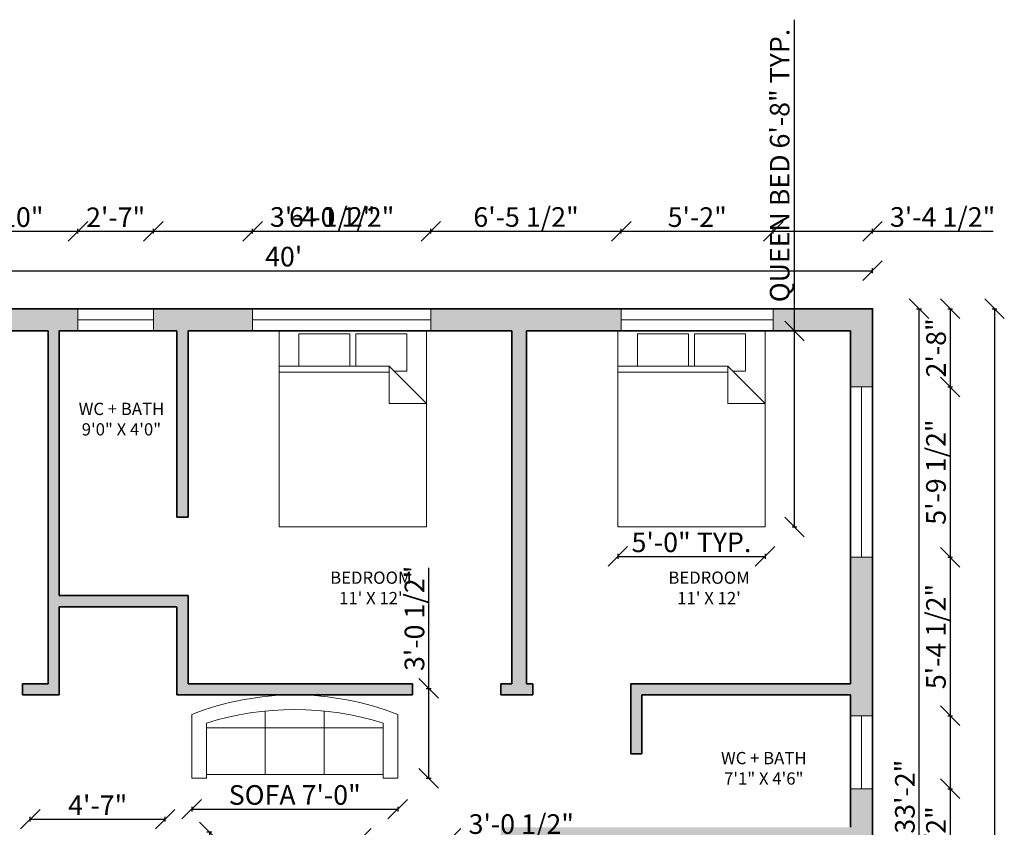
# Model space of a CAD drawing. Units: inches. Extents: x 2561 to 3163, y 493 to 1211.
# Tile 8 of 8: x 2762 to 3163, y 882 to 1211. Entities that reach past the tile are written whole.
import ezdxf

# ---------------------------------------------------------------- set-up
doc = ezdxf.new("R2010")
doc.units = ezdxf.units.IN
for name, color, linetype, lineweight in [('A-ANNO-DIMS', 2, 'Continuous', 18), ('A-AREA-IDEN', 7, 'Continuous', 18), ('A-FURN', 8, 'Continuous', 18), ('A-GLAZ', 4, 'Continuous', 18), ('A-WALL', 7, 'Continuous', 35), ('A-WALL-PATT', 24, 'Continuous', 13)]:
    doc.layers.add(name, color=color, linetype=linetype, lineweight=lineweight)
doc.styles.get("Standard").update_dxf_attribs({"font": 'arial.ttf'})
doc.dimstyles.new('ISO-25', dxfattribs={"dimtxt": 8, "dimasz": 8, "dimexe": 1, "dimexo": 1, "dimtad": 1, "dimlunit": 3, "dimtxsty": 'Standard', "dimblk": 'OBLIQUE', "dimcen": 2.5, "dimadec": 0, "dimazin": 0, "dimtfac": 1, "dimtmove": 0, "dimatfit": 3, "dimfxl": 1, "dimfxlon": 1, "dimarcsym": 0})

# ---------------------------------------------------------------- blocks, each defined once
blk = doc.blocks.new('Sofa - Roundback 7 ft.')
for p, q in [((-12.00002, -32.4421), (-12.00003, -6.5971)), ((11.99997, -32.4421), (11.99998, -6.5971)), ((-36.000027, -34), (-36.000027, -11.4696)), ((35.99998, -34), (35.99998, -11.4696)), ((-35.999844, -13.3819), (35.9998, -13.3819)), ((-36.000027, -32.4421), (35.99998, -32.4421))]:
    blk.add_line(p, q)
for points in [[(-36.000027, -34), (-42.000027, -34), (-42.000027, -8)], [(41.99998, -8), (41.99998, -34), (35.99998, -34)]]:
    blk.add_lwpolyline(points)
for centre, radius, start, end in [((0, -114.25), 114.25, 68.43141, 111.5686), ((-0.00001, -127.1968), 121.1968, 72.72033, 107.2797)]:
    blk.add_arc(centre, radius, start, end)
blk = doc.blocks.new('Bed - Queen')
for p, q in [((0, -80.00003), (0, 0)), ((0, 0), (59.99999, 0)), ((59.99999, 0), (59.99999, -80.00003)), ((7.99999, -1.2), (28.79998, -1.2)), ((7.99999, -14.4), (7.99999, -1.2)), ((28.79998, -1.2), (28.79998, -14.4)), ((31.19999, -1.2), (51.99999, -1.2)), ((31.19999, -14.4), (31.19999, -1.2)), ((51.99999, -1.2), (51.99999, -16.4)), ((0, -14.4), (44.8, -14.4)), ((59.99999, -29.6), (44.8, -14.4)), ((44.8, -14.4), (44.8, -29.6)), ((44.8, -16.8), (0, -16.8)), ((51.99999, -16.4), (46.79936, -16.4)), ((44.8, -29.6), (59.99999, -29.6)), ((59.99999, -80.00003), (0, -80.00003))]:
    blk.add_line(p, q)
blk = doc.blocks.new('_Oblique')
at = {"color": 0, "linetype": 'ByBlock', "lineweight": -2}
blk.add_line((-0.5, -0.5), (0.5, 0.5), dxfattribs=at)
blk = doc.blocks.new('*D8')
at = {"layer": 'A-ANNO-DIMS', "color": 0, "lineweight": -2, "transparency": 16777216}
for p, q in [((2629.27, 1107.6), (2629.27, 1109.6)), ((2629.27, 1108.6), (3109.27, 1108.6)), ((3109.27, 1107.6), (3109.27, 1109.6))]:
    blk.add_line(p, q, dxfattribs=at)
at = {"layer": 'Defpoints', "color": 0, "transparency": 16777216}
for p in [(3109.27, 1108.6), (2629.27, 1093.07), (3109.27, 1093.07)]:
    blk.add_point(p, dxfattribs=at)
at = {"layer": 'A-ANNO-DIMS', "color": 0, "lineweight": -2, "transparency": 16777216, "xscale": 8, "yscale": 8, "zscale": 8, "rotation": 180}
blk.add_blockref('_Oblique', (2629.27, 1108.6), dxfattribs=at)
at = {"layer": 'A-ANNO-DIMS', "color": 0, "lineweight": -2, "transparency": 16777216, "xscale": 8, "yscale": 8, "zscale": 8}
blk.add_blockref('_Oblique', (3109.27, 1108.6), dxfattribs=at)
at = {"layer": 'A-ANNO-DIMS', "color": 0, "transparency": 16777216, "insert": (2869.27, 1113.31), "char_height": 8, "attachment_point": 5}
blk.add_mtext("40'", dxfattribs=at)
blk = doc.blocks.new('*D10')
at = {"layer": 'A-ANNO-DIMS', "color": 0, "lineweight": -2, "transparency": 16777216}
for p, q in [((3127.21, 1093.07), (3129.21, 1093.07)), ((3128.21, 1093.07), (3128.21, 695.07)), ((3127.21, 695.07), (3129.21, 695.07))]:
    blk.add_line(p, q, dxfattribs=at)
at = {"layer": 'Defpoints', "color": 0, "transparency": 16777216}
for p in [(3109.27, 1093.07), (3109.27, 695.07), (3128.21, 695.07)]:
    blk.add_point(p, dxfattribs=at)
at = {"layer": 'A-ANNO-DIMS', "color": 0, "lineweight": -2, "transparency": 16777216, "xscale": 8, "yscale": 8, "zscale": 8}
for p, rotation in [((3128.21, 1093.07), 90), ((3128.21, 695.07), 270)]:
    blk.add_blockref('_Oblique', p, dxfattribs=dict(at, rotation=rotation))
at = {"layer": 'A-ANNO-DIMS', "color": 0, "transparency": 16777216, "insert": (3123.5, 894.07), "char_height": 8, "attachment_point": 5, "rotation": 90}
blk.add_mtext('33\'-2"', dxfattribs=at)
blk = doc.blocks.new('*D13')
at = {"layer": 'A-ANNO-DIMS', "color": 0, "lineweight": -2, "transparency": 16777216}
for p, q in [((3157.99, 1093.07), (3159.99, 1093.07)), ((3158.99, 1093.07), (3158.99, 529.07)), ((3157.99, 529.07), (3159.99, 529.07))]:
    blk.add_line(p, q, dxfattribs=at)
at = {"layer": 'Defpoints', "color": 0, "transparency": 16777216}
for p in [(3109.27, 1093.07), (3109.27, 529.07), (3158.99, 529.07)]:
    blk.add_point(p, dxfattribs=at)
at = {"layer": 'A-ANNO-DIMS', "color": 0, "lineweight": -2, "transparency": 16777216, "xscale": 8, "yscale": 8, "zscale": 8}
for p, rotation in [((3158.99, 1093.07), 90), ((3158.99, 529.07), 270)]:
    blk.add_blockref('_Oblique', p, dxfattribs=dict(at, rotation=rotation))
at = {"layer": 'A-ANNO-DIMS', "color": 0, "transparency": 16777216, "insert": (3154.37, 811.07), "char_height": 8, "attachment_point": 5, "rotation": 90}
blk.add_mtext("47'", dxfattribs=at)
blk = doc.blocks.new('*D17')
at = {"layer": 'A-ANNO-DIMS', "color": 0, "lineweight": -2, "transparency": 16777216}
for p, q in [((2571.63, 1093.07), (2569.63, 1093.07)), ((2570.63, 1093.07), (2570.63, 529.07)), ((2571.63, 529.07), (2569.63, 529.07))]:
    blk.add_line(p, q, dxfattribs=at)
at = {"layer": 'Defpoints', "color": 0, "transparency": 16777216}
for p in [(2629.27, 1093.07), (2570.63, 529.07), (3109.27, 529.07)]:
    blk.add_point(p, dxfattribs=at)
at = {"layer": 'A-ANNO-DIMS', "color": 0, "lineweight": -2, "transparency": 16777216, "xscale": 8, "yscale": 8, "zscale": 8}
for p, rotation in [((2570.63, 1093.07), 90), ((2570.63, 529.07), 270)]:
    blk.add_blockref('_Oblique', p, dxfattribs=dict(at, rotation=rotation))
at = {"layer": 'A-ANNO-DIMS', "color": 0, "transparency": 16777216, "insert": (2566, 811.07), "char_height": 8, "attachment_point": 5, "rotation": 90}
blk.add_mtext("47'", dxfattribs=at)
blk = doc.blocks.new('*D18')
at = {"layer": 'A-ANNO-DIMS', "color": 0, "lineweight": -2, "transparency": 16777216}
for p, q in [((3077.47, 1084.07), (3077.47, 1211)), ((3076.47, 1084.07), (3078.47, 1084.07)), ((3077.47, 1004.07), (3077.47, 1084.07)), ((3076.47, 1004.07), (3078.47, 1004.07))]:
    blk.add_line(p, q, dxfattribs=at)
at = {"layer": 'Defpoints', "color": 0, "transparency": 16777216}
for p in [(3065.47, 1084.07), (3077.47, 1084.07), (3065.47, 1004.07)]:
    blk.add_point(p, dxfattribs=at)
at = {"layer": 'A-ANNO-DIMS', "color": 0, "lineweight": -2, "transparency": 16777216, "xscale": 8, "yscale": 8, "zscale": 8}
for p, rotation in [((3077.47, 1084.07), 90), ((3077.47, 1004.07), 270)]:
    blk.add_blockref('_Oblique', p, dxfattribs=dict(at, rotation=rotation))
at = {"layer": 'A-ANNO-DIMS', "color": 0, "transparency": 16777216, "insert": (3072.47, 1151.53), "char_height": 8, "attachment_point": 5, "rotation": 90}
blk.add_mtext('QUEEN BED 6\'-8" TYP.', dxfattribs=at)
blk = doc.blocks.new('*D19')
at = {"layer": 'A-ANNO-DIMS', "color": 0, "lineweight": -2, "transparency": 16777216}
for p, q in [((3005.47, 993.07), (3005.47, 991.07)), ((3005.47, 992.07), (3065.47, 992.07)), ((3065.47, 993.07), (3065.47, 991.07))]:
    blk.add_line(p, q, dxfattribs=at)
at = {"layer": 'Defpoints', "color": 0, "transparency": 16777216}
for p in [(3005.47, 1004.07), (3065.47, 1004.07), (3065.47, 992.07)]:
    blk.add_point(p, dxfattribs=at)
at = {"layer": 'A-ANNO-DIMS', "color": 0, "lineweight": -2, "transparency": 16777216, "xscale": 8, "yscale": 8, "zscale": 8, "rotation": 180}
blk.add_blockref('_Oblique', (3005.47, 992.07), dxfattribs=at)
at = {"layer": 'A-ANNO-DIMS', "color": 0, "lineweight": -2, "transparency": 16777216, "xscale": 8, "yscale": 8, "zscale": 8}
blk.add_blockref('_Oblique', (3065.47, 992.07), dxfattribs=at)
at = {"layer": 'A-ANNO-DIMS', "color": 0, "transparency": 16777216, "insert": (3035.47, 996.78), "char_height": 8, "attachment_point": 5}
blk.add_mtext('5\'-0" TYP.', dxfattribs=at)
blk = doc.blocks.new('*D22')
at = {"layer": 'A-ANNO-DIMS', "color": 0, "lineweight": -2, "transparency": 16777216}
for p, q in [((2831.77, 889.97), (2831.77, 887.97)), ((2831.77, 888.97), (2915.77, 888.97)), ((2915.77, 889.97), (2915.77, 887.97))]:
    blk.add_line(p, q, dxfattribs=at)
at = {"layer": 'Defpoints', "color": 0, "transparency": 16777216}
for p in [(2831.77, 901.57), (2915.77, 901.57), (2915.77, 888.97)]:
    blk.add_point(p, dxfattribs=at)
at = {"layer": 'A-ANNO-DIMS', "color": 0, "lineweight": -2, "transparency": 16777216, "xscale": 8, "yscale": 8, "zscale": 8, "rotation": 180}
blk.add_blockref('_Oblique', (2831.77, 888.97), dxfattribs=at)
at = {"layer": 'A-ANNO-DIMS', "color": 0, "lineweight": -2, "transparency": 16777216, "xscale": 8, "yscale": 8, "zscale": 8}
blk.add_blockref('_Oblique', (2915.77, 888.97), dxfattribs=at)
at = {"layer": 'A-ANNO-DIMS', "color": 0, "transparency": 16777216, "insert": (2873.77, 893.73), "char_height": 8, "attachment_point": 5}
blk.add_mtext('SOFA 7\'-0"', dxfattribs=at)
blk = doc.blocks.new('*D23')
at = {"layer": 'A-ANNO-DIMS', "color": 0, "lineweight": -2, "transparency": 16777216}
for p, q in [((2928.37, 938.24), (2928.37, 987.39)), ((2927.37, 938.24), (2929.37, 938.24)), ((2928.37, 901.57), (2928.37, 938.24)), ((2927.37, 901.57), (2929.37, 901.57))]:
    blk.add_line(p, q, dxfattribs=at)
at = {"layer": 'Defpoints', "color": 0, "transparency": 16777216}
for p in [(2915.77, 938.24), (2928.37, 938.24), (2915.77, 901.57)]:
    blk.add_point(p, dxfattribs=at)
at = {"layer": 'A-ANNO-DIMS', "color": 0, "lineweight": -2, "transparency": 16777216, "xscale": 8, "yscale": 8, "zscale": 8}
for p, rotation in [((2928.37, 938.24), 90), ((2928.37, 901.57), 270)]:
    blk.add_blockref('_Oblique', p, dxfattribs=dict(at, rotation=rotation))
at = {"layer": 'A-ANNO-DIMS', "color": 0, "transparency": 16777216, "insert": (2923.61, 966.81), "char_height": 8, "attachment_point": 5, "rotation": 90}
blk.add_mtext('3\'-0 1/2"', dxfattribs=at)
blk = doc.blocks.new('*D24')
at = {"layer": 'A-ANNO-DIMS', "color": 0, "lineweight": -2, "transparency": 16777216}
for p, q in [((2839.96, 879.66), (2837.96, 879.66)), ((2838.96, 879.66), (2838.96, 819.66)), ((2839.96, 819.66), (2837.96, 819.66)), ((2838.96, 819.66), (2838.96, 750.44))]:
    blk.add_line(p, q, dxfattribs=at)
at = {"layer": 'Defpoints', "color": 0, "transparency": 16777216}
for p in [(2847.96, 879.66), (2838.96, 819.66), (2847.96, 819.66)]:
    blk.add_point(p, dxfattribs=at)
at = {"layer": 'A-ANNO-DIMS', "color": 0, "lineweight": -2, "transparency": 16777216, "xscale": 8, "yscale": 8, "zscale": 8}
for p, rotation in [((2838.96, 879.66), 90), ((2838.96, 819.66), 270)]:
    blk.add_blockref('_Oblique', p, dxfattribs=dict(at, rotation=rotation))
at = {"layer": 'A-ANNO-DIMS', "color": 0, "transparency": 16777216, "insert": (2834.25, 781.05), "char_height": 8, "attachment_point": 5, "rotation": 90}
blk.add_mtext('TABLE 5\'-0"', dxfattribs=at)
blk = doc.blocks.new('*D27')
at = {"layer": 'A-ANNO-DIMS', "color": 0, "lineweight": -2, "transparency": 16777216}
for p, q in [((2900.86, 876.1), (2900.86, 878.1)), ((2900.86, 877.1), (2937.53, 877.1)), ((2937.53, 876.1), (2937.53, 878.1)), ((2937.53, 877.1), (2986.68, 877.1))]:
    blk.add_line(p, q, dxfattribs=at)
at = {"layer": 'Defpoints', "color": 0, "transparency": 16777216}
for p in [(2937.53, 877.1), (2900.86, 868.1), (2937.53, 868.1)]:
    blk.add_point(p, dxfattribs=at)
at = {"layer": 'A-ANNO-DIMS', "color": 0, "lineweight": -2, "transparency": 16777216, "xscale": 8, "yscale": 8, "zscale": 8, "rotation": 180}
blk.add_blockref('_Oblique', (2900.86, 877.1), dxfattribs=at)
at = {"layer": 'A-ANNO-DIMS', "color": 0, "lineweight": -2, "transparency": 16777216, "xscale": 8, "yscale": 8, "zscale": 8}
blk.add_blockref('_Oblique', (2937.53, 877.1), dxfattribs=at)
at = {"layer": 'A-ANNO-DIMS', "color": 0, "transparency": 16777216, "insert": (2966.11, 881.86), "char_height": 8, "attachment_point": 5}
blk.add_mtext('3\'-0 1/2"', dxfattribs=at)
blk = doc.blocks.new('*D29')
at = {"layer": 'A-ANNO-DIMS', "color": 0, "lineweight": -2, "transparency": 16777216}
for p, q in [((2765.96, 883.89), (2765.96, 885.89)), ((2765.96, 884.89), (2820.96, 884.89)), ((2820.96, 883.89), (2820.96, 885.89))]:
    blk.add_line(p, q, dxfattribs=at)
at = {"layer": 'Defpoints', "color": 0, "transparency": 16777216}
for p in [(2820.96, 884.89), (2765.96, 871.24), (2820.96, 871.24)]:
    blk.add_point(p, dxfattribs=at)
at = {"layer": 'A-ANNO-DIMS', "color": 0, "lineweight": -2, "transparency": 16777216, "xscale": 8, "yscale": 8, "zscale": 8, "rotation": 180}
blk.add_blockref('_Oblique', (2765.96, 884.89), dxfattribs=at)
at = {"layer": 'A-ANNO-DIMS', "color": 0, "lineweight": -2, "transparency": 16777216, "xscale": 8, "yscale": 8, "zscale": 8}
blk.add_blockref('_Oblique', (2820.96, 884.89), dxfattribs=at)
at = {"layer": 'A-ANNO-DIMS', "color": 0, "transparency": 16777216, "insert": (2793.46, 889.52), "char_height": 8, "attachment_point": 5}
blk.add_mtext('4\'-7"', dxfattribs=at)
blk = doc.blocks.new('*D35')
at = {"layer": 'A-ANNO-DIMS', "color": 0, "lineweight": -2, "transparency": 16777216}
for p, q in [((2727.19, 1123.72), (2727.19, 1125.72)), ((2727.19, 1124.72), (2785.37, 1124.72)), ((2785.37, 1123.72), (2785.37, 1125.72))]:
    blk.add_line(p, q, dxfattribs=at)
at = {"layer": 'Defpoints', "color": 0, "transparency": 16777216}
for p in [(2785.37, 1124.72), (2727.19, 1093.07), (2785.37, 1093.07)]:
    blk.add_point(p, dxfattribs=at)
at = {"layer": 'A-ANNO-DIMS', "color": 0, "lineweight": -2, "transparency": 16777216, "xscale": 8, "yscale": 8, "zscale": 8, "rotation": 180}
blk.add_blockref('_Oblique', (2727.19, 1124.72), dxfattribs=at)
at = {"layer": 'A-ANNO-DIMS', "color": 0, "lineweight": -2, "transparency": 16777216, "xscale": 8, "yscale": 8, "zscale": 8}
blk.add_blockref('_Oblique', (2785.37, 1124.72), dxfattribs=at)
at = {"layer": 'A-ANNO-DIMS', "color": 0, "transparency": 16777216, "insert": (2756.28, 1129.43), "char_height": 8, "attachment_point": 5}
blk.add_mtext('4\'-10"', dxfattribs=at)
blk = doc.blocks.new('*D36')
at = {"layer": 'A-ANNO-DIMS', "color": 0, "lineweight": -2, "transparency": 16777216}
for p, q in [((2785.37, 1123.72), (2785.37, 1125.72)), ((2785.37, 1124.72), (2816.17, 1124.72)), ((2816.17, 1123.72), (2816.17, 1125.72))]:
    blk.add_line(p, q, dxfattribs=at)
at = {"layer": 'Defpoints', "color": 0, "transparency": 16777216}
for p in [(2816.17, 1124.72), (2785.37, 1093.07), (2816.17, 1093.07)]:
    blk.add_point(p, dxfattribs=at)
at = {"layer": 'A-ANNO-DIMS', "color": 0, "lineweight": -2, "transparency": 16777216, "xscale": 8, "yscale": 8, "zscale": 8, "rotation": 180}
blk.add_blockref('_Oblique', (2785.37, 1124.72), dxfattribs=at)
at = {"layer": 'A-ANNO-DIMS', "color": 0, "lineweight": -2, "transparency": 16777216, "xscale": 8, "yscale": 8, "zscale": 8}
blk.add_blockref('_Oblique', (2816.17, 1124.72), dxfattribs=at)
at = {"layer": 'A-ANNO-DIMS', "color": 0, "transparency": 16777216, "insert": (2800.77, 1129.36), "char_height": 8, "attachment_point": 5}
blk.add_mtext('2\'-7"', dxfattribs=at)
blk = doc.blocks.new('*D37')
at = {"layer": 'A-ANNO-DIMS', "color": 0, "lineweight": -2, "transparency": 16777216}
for p, q in [((2816.17, 1123.72), (2816.17, 1125.72)), ((2816.17, 1124.72), (2856.57, 1124.72)), ((2856.57, 1123.72), (2856.57, 1125.72)), ((2856.57, 1124.72), (2905.72, 1124.72))]:
    blk.add_line(p, q, dxfattribs=at)
at = {"layer": 'Defpoints', "color": 0, "transparency": 16777216}
for p in [(2856.57, 1124.72), (2816.17, 1093.07), (2856.57, 1093.07)]:
    blk.add_point(p, dxfattribs=at)
at = {"layer": 'A-ANNO-DIMS', "color": 0, "lineweight": -2, "transparency": 16777216, "xscale": 8, "yscale": 8, "zscale": 8, "rotation": 180}
blk.add_blockref('_Oblique', (2816.17, 1124.72), dxfattribs=at)
at = {"layer": 'A-ANNO-DIMS', "color": 0, "lineweight": -2, "transparency": 16777216, "xscale": 8, "yscale": 8, "zscale": 8}
blk.add_blockref('_Oblique', (2856.57, 1124.72), dxfattribs=at)
at = {"layer": 'A-ANNO-DIMS', "color": 0, "transparency": 16777216, "insert": (2885.14, 1129.48), "char_height": 8, "attachment_point": 5}
blk.add_mtext('3\'-4 1/2"', dxfattribs=at)
blk = doc.blocks.new('*D38')
at = {"layer": 'A-ANNO-DIMS', "color": 0, "lineweight": -2, "transparency": 16777216}
for p, q in [((2856.57, 1123.72), (2856.57, 1125.72)), ((2856.57, 1124.72), (2929.24, 1124.72)), ((2929.24, 1123.72), (2929.24, 1125.72))]:
    blk.add_line(p, q, dxfattribs=at)
at = {"layer": 'Defpoints', "color": 0, "transparency": 16777216}
for p in [(2929.24, 1124.72), (2856.57, 1093.07), (2929.24, 1093.07)]:
    blk.add_point(p, dxfattribs=at)
at = {"layer": 'A-ANNO-DIMS', "color": 0, "lineweight": -2, "transparency": 16777216, "xscale": 8, "yscale": 8, "zscale": 8, "rotation": 180}
blk.add_blockref('_Oblique', (2856.57, 1124.72), dxfattribs=at)
at = {"layer": 'A-ANNO-DIMS', "color": 0, "lineweight": -2, "transparency": 16777216, "xscale": 8, "yscale": 8, "zscale": 8}
blk.add_blockref('_Oblique', (2929.24, 1124.72), dxfattribs=at)
at = {"layer": 'A-ANNO-DIMS', "color": 0, "transparency": 16777216, "insert": (2892.9, 1129.48), "char_height": 8, "attachment_point": 5}
blk.add_mtext('6\'-0 1/2"', dxfattribs=at)
blk = doc.blocks.new('*D39')
at = {"layer": 'A-ANNO-DIMS', "color": 0, "lineweight": -2, "transparency": 16777216}
for p, q in [((2929.24, 1123.72), (2929.24, 1125.72)), ((2929.24, 1124.72), (3006.87, 1124.72)), ((3006.87, 1123.72), (3006.87, 1125.72))]:
    blk.add_line(p, q, dxfattribs=at)
at = {"layer": 'Defpoints', "color": 0, "transparency": 16777216}
for p in [(3006.87, 1124.72), (2929.24, 1093.07), (3006.87, 1093.07)]:
    blk.add_point(p, dxfattribs=at)
at = {"layer": 'A-ANNO-DIMS', "color": 0, "lineweight": -2, "transparency": 16777216, "xscale": 8, "yscale": 8, "zscale": 8, "rotation": 180}
blk.add_blockref('_Oblique', (2929.24, 1124.72), dxfattribs=at)
at = {"layer": 'A-ANNO-DIMS', "color": 0, "lineweight": -2, "transparency": 16777216, "xscale": 8, "yscale": 8, "zscale": 8}
blk.add_blockref('_Oblique', (3006.87, 1124.72), dxfattribs=at)
at = {"layer": 'A-ANNO-DIMS', "color": 0, "transparency": 16777216, "insert": (2968.05, 1129.48), "char_height": 8, "attachment_point": 5}
blk.add_mtext('6\'-5 1/2"', dxfattribs=at)
blk = doc.blocks.new('*D40')
at = {"layer": 'A-ANNO-DIMS', "color": 0, "lineweight": -2, "transparency": 16777216}
for p, q in [((3006.87, 1123.72), (3006.87, 1125.72)), ((3006.87, 1124.72), (3068.8, 1124.72)), ((3068.8, 1123.72), (3068.8, 1125.72))]:
    blk.add_line(p, q, dxfattribs=at)
at = {"layer": 'Defpoints', "color": 0, "transparency": 16777216}
for p in [(3068.8, 1124.72), (3006.87, 1093.07), (3068.8, 1093.07)]:
    blk.add_point(p, dxfattribs=at)
at = {"layer": 'A-ANNO-DIMS', "color": 0, "lineweight": -2, "transparency": 16777216, "xscale": 8, "yscale": 8, "zscale": 8, "rotation": 180}
blk.add_blockref('_Oblique', (3006.87, 1124.72), dxfattribs=at)
at = {"layer": 'A-ANNO-DIMS', "color": 0, "lineweight": -2, "transparency": 16777216, "xscale": 8, "yscale": 8, "zscale": 8}
blk.add_blockref('_Oblique', (3068.8, 1124.72), dxfattribs=at)
at = {"layer": 'A-ANNO-DIMS', "color": 0, "transparency": 16777216, "insert": (3037.83, 1129.43), "char_height": 8, "attachment_point": 5}
blk.add_mtext('5\'-2"', dxfattribs=at)
blk = doc.blocks.new('*D41')
at = {"layer": 'A-ANNO-DIMS', "color": 0, "lineweight": -2, "transparency": 16777216}
for p, q in [((3068.8, 1123.72), (3068.8, 1125.72)), ((3068.8, 1124.72), (3109.27, 1124.72)), ((3109.27, 1123.72), (3109.27, 1125.72)), ((3109.27, 1124.72), (3158.43, 1124.72))]:
    blk.add_line(p, q, dxfattribs=at)
at = {"layer": 'Defpoints', "color": 0, "transparency": 16777216}
for p in [(3109.27, 1124.72), (3068.8, 1093.07), (3109.27, 1093.07)]:
    blk.add_point(p, dxfattribs=at)
at = {"layer": 'A-ANNO-DIMS', "color": 0, "lineweight": -2, "transparency": 16777216, "xscale": 8, "yscale": 8, "zscale": 8, "rotation": 180}
blk.add_blockref('_Oblique', (3068.8, 1124.72), dxfattribs=at)
at = {"layer": 'A-ANNO-DIMS', "color": 0, "lineweight": -2, "transparency": 16777216, "xscale": 8, "yscale": 8, "zscale": 8}
blk.add_blockref('_Oblique', (3109.27, 1124.72), dxfattribs=at)
at = {"layer": 'A-ANNO-DIMS', "color": 0, "transparency": 16777216, "insert": (3137.85, 1129.48), "char_height": 8, "attachment_point": 5}
blk.add_mtext('3\'-4 1/2"', dxfattribs=at)
blk = doc.blocks.new('*D51')
at = {"layer": 'A-ANNO-DIMS', "color": 0, "lineweight": -2, "transparency": 16777216}
for p, q in [((3139.92, 1093.07), (3141.92, 1093.07)), ((3140.92, 1093.07), (3140.92, 1061.19)), ((3139.92, 1061.19), (3141.92, 1061.19))]:
    blk.add_line(p, q, dxfattribs=at)
at = {"layer": 'Defpoints', "color": 0, "transparency": 16777216}
for p in [(3109.27, 1093.07), (3109.27, 1061.19), (3140.92, 1061.19)]:
    blk.add_point(p, dxfattribs=at)
at = {"layer": 'A-ANNO-DIMS', "color": 0, "lineweight": -2, "transparency": 16777216, "xscale": 8, "yscale": 8, "zscale": 8}
for p, rotation in [((3140.92, 1093.07), 90), ((3140.92, 1061.19), 270)]:
    blk.add_blockref('_Oblique', p, dxfattribs=dict(at, rotation=rotation))
at = {"layer": 'A-ANNO-DIMS', "color": 0, "transparency": 16777216, "insert": (3136.21, 1077.13), "char_height": 8, "attachment_point": 5, "rotation": 90}
blk.add_mtext('2\'-8"', dxfattribs=at)
blk = doc.blocks.new('*D52')
at = {"layer": 'A-ANNO-DIMS', "color": 0, "lineweight": -2, "transparency": 16777216}
for p, q in [((3139.92, 1061.19), (3141.92, 1061.19)), ((3140.92, 1061.19), (3140.92, 991.72)), ((3139.92, 991.72), (3141.92, 991.72))]:
    blk.add_line(p, q, dxfattribs=at)
at = {"layer": 'Defpoints', "color": 0, "transparency": 16777216}
for p in [(3109.27, 1061.19), (3109.27, 991.72), (3140.92, 991.72)]:
    blk.add_point(p, dxfattribs=at)
at = {"layer": 'A-ANNO-DIMS', "color": 0, "lineweight": -2, "transparency": 16777216, "xscale": 8, "yscale": 8, "zscale": 8}
for p, rotation in [((3140.92, 1061.19), 90), ((3140.92, 991.72), 270)]:
    blk.add_blockref('_Oblique', p, dxfattribs=dict(at, rotation=rotation))
at = {"layer": 'A-ANNO-DIMS', "color": 0, "transparency": 16777216, "insert": (3136.16, 1026.46), "char_height": 8, "attachment_point": 5, "rotation": 90}
blk.add_mtext('5\'-9 1/2"', dxfattribs=at)
blk = doc.blocks.new('*D53')
at = {"layer": 'A-ANNO-DIMS', "color": 0, "lineweight": -2, "transparency": 16777216}
for p, q in [((3139.92, 991.72), (3141.92, 991.72)), ((3140.92, 991.72), (3140.92, 927.07)), ((3139.92, 927.07), (3141.92, 927.07))]:
    blk.add_line(p, q, dxfattribs=at)
at = {"layer": 'Defpoints', "color": 0, "transparency": 16777216}
for p in [(3109.27, 991.72), (3109.27, 927.07), (3140.92, 927.07)]:
    blk.add_point(p, dxfattribs=at)
at = {"layer": 'A-ANNO-DIMS', "color": 0, "lineweight": -2, "transparency": 16777216, "xscale": 8, "yscale": 8, "zscale": 8}
for p, rotation in [((3140.92, 991.72), 90), ((3140.92, 927.07), 270)]:
    blk.add_blockref('_Oblique', p, dxfattribs=dict(at, rotation=rotation))
at = {"layer": 'A-ANNO-DIMS', "color": 0, "transparency": 16777216, "insert": (3136.16, 959.4), "char_height": 8, "attachment_point": 5, "rotation": 90}
blk.add_mtext('5\'-4 1/2"', dxfattribs=at)
blk = doc.blocks.new('*D54')
at = {"layer": 'A-ANNO-DIMS', "color": 0, "lineweight": -2, "transparency": 16777216}
for p, q in [((3139.92, 927.07), (3141.92, 927.07)), ((3140.92, 927.07), (3140.92, 897.33)), ((3139.92, 897.33), (3141.92, 897.33)), ((3140.92, 897.33), (3140.92, 848.03))]:
    blk.add_line(p, q, dxfattribs=at)
at = {"layer": 'Defpoints', "color": 0, "transparency": 16777216}
for p in [(3109.27, 927.07), (3109.27, 897.33), (3140.92, 897.33)]:
    blk.add_point(p, dxfattribs=at)
at = {"layer": 'A-ANNO-DIMS', "color": 0, "lineweight": -2, "transparency": 16777216, "xscale": 8, "yscale": 8, "zscale": 8}
for p, rotation in [((3140.92, 927.07), 90), ((3140.92, 897.33), 270)]:
    blk.add_blockref('_Oblique', p, dxfattribs=dict(at, rotation=rotation))
at = {"layer": 'A-ANNO-DIMS', "color": 0, "transparency": 16777216, "insert": (3136.16, 868.68), "char_height": 8, "attachment_point": 5, "rotation": 90}
blk.add_mtext('2\'-5 1/2"', dxfattribs=at)
blk = doc.blocks.new('*D55')
at = {"layer": 'A-ANNO-DIMS', "color": 0, "lineweight": -2, "transparency": 16777216}
for p, q in [((3139.92, 897.33), (3141.92, 897.33)), ((3140.92, 897.33), (3140.92, 805.79)), ((3139.92, 805.79), (3141.92, 805.79))]:
    blk.add_line(p, q, dxfattribs=at)
at = {"layer": 'Defpoints', "color": 0, "transparency": 16777216}
for p in [(3109.27, 897.33), (3109.27, 805.79), (3140.92, 805.79)]:
    blk.add_point(p, dxfattribs=at)
at = {"layer": 'A-ANNO-DIMS', "color": 0, "lineweight": -2, "transparency": 16777216, "xscale": 8, "yscale": 8, "zscale": 8}
for p, rotation in [((3140.92, 897.33), 90), ((3140.92, 805.79), 270)]:
    blk.add_blockref('_Oblique', p, dxfattribs=dict(at, rotation=rotation))
at = {"layer": 'A-ANNO-DIMS', "color": 0, "transparency": 16777216, "insert": (3136.16, 851.56), "char_height": 8, "attachment_point": 5, "rotation": 90}
blk.add_mtext('7\'-7 1/2"', dxfattribs=at)

msp = doc.modelspace()

# ---------------------------------------------------------------- hatches: boundary and pattern name
at = {"layer": 'A-WALL-PATT'}
h = msp.add_hatch(color=256, dxfattribs=at)
h.dxf.hatch_style = 1
h.paths.add_polyline_path([(2665.022, 1093.069), (2629.274, 1093.069), (2629.274, 1056.034), (2638.274, 1056.034), (2638.274, 1084.069), (2665.022, 1084.069)])
h.paths.add_polyline_path([(2785.37, 1093.069), (2727.193, 1093.069), (2727.193, 1084.069), (2773.274, 1084.069), (2773.274, 940.069), (2762.774, 940.069), (2762.774, 935.569), (2777.774, 935.569), (2777.774, 971.569), (2825.774, 971.569), (2825.774, 935.569), (2921.774, 935.569), (2921.774, 940.069), (2830.274, 940.069), (2830.274, 976.069), (2777.774, 976.069), (2777.774, 1084.069), (2785.37, 1084.069)])
h.paths.add_polyline_path([(2856.568, 1093.069), (2816.168, 1093.069), (2816.168, 1084.069), (2825.774, 1084.069), (2825.774, 1008.069), (2830.274, 1008.069), (2830.274, 1084.069), (2856.568, 1084.069)], flags=17)
h.paths.add_polyline_path([(3006.866, 1093.069), (2929.24, 1093.069), (2929.24, 1084.069), (2962.274, 1084.069), (2962.274, 940.069), (2957.774, 940.069), (2957.774, 935.569), (2970.774, 935.569), (2970.774, 940.069), (2968.274, 940.069), (2968.274, 1084.069), (3006.866, 1084.069)])
h.paths.add_polyline_path([(3109.274, 1093.069), (3068.804, 1093.069), (3068.804, 1084.069), (3100.274, 1084.069), (3100.274, 1061.194), (3109.274, 1061.194)])
h.paths.add_polyline_path([(3109.274, 991.723), (3100.274, 991.723), (3100.274, 940.069), (3010.774, 940.069), (3010.774, 935.569), (3010.774, 911.569), (3015.274, 911.569), (3015.274, 935.569), (3100.274, 935.569), (3100.274, 927.07), (3109.274, 927.07)])
h.paths.add_polyline_path([(3109.274, 897.327), (3100.274, 897.327), (3100.274, 881.569), (2957.774, 881.569), (2957.774, 872.569), (3100.274, 872.569), (3100.274, 805.791), (3109.274, 805.791)])
h.paths.add_polyline_path([(2638.274, 982.372), (2629.274, 982.372), (2629.274, 927.027), (2638.274, 927.027), (2638.274, 935.569), (2722.274, 935.569), (2722.274, 919.569), (2726.774, 919.569), (2726.774, 940.069), (2638.274, 940.069)])
h.paths.add_polyline_path([(2638.274, 883.069), (2726.774, 883.069), (2726.774, 887.569), (2638.274, 887.569), (2638.274, 897.75), (2629.274, 897.75), (2629.274, 856.591), (2638.274, 856.591)])
h.paths.add_polyline_path([(2726.774, 851.069), (2722.274, 851.069), (2722.274, 772.069), (2638.274, 772.069), (2638.274, 802.178), (2629.274, 802.178), (2629.274, 725.136), (2638.274, 725.136), (2638.274, 767.569), (2726.774, 767.569)])
h.paths.add_polyline_path([(2638.274, 659.235), (2629.274, 659.235), (2629.274, 614.569), (2638.274, 614.569)])
h.paths.add_polyline_path([(2664.613, 623.569), (2638.274, 623.569), (2638.274, 614.569), (2664.613, 614.569)])
h.paths.add_polyline_path([(2787.908, 623.569), (2777.774, 623.569), (2777.774, 767.569), (2825.774, 767.569), (2825.774, 659.569), (2830.274, 659.569), (2830.274, 767.569), (2836.774, 767.569), (2836.774, 772.069), (2766.674, 772.069), (2766.674, 767.569), (2773.274, 767.569), (2773.274, 623.569), (2722.435, 623.569), (2722.435, 614.569), (2787.908, 614.569)])
h.paths.add_polyline_path([(2883.664, 623.569), (2867.474, 623.569), (2818.294, 623.569), (2818.294, 614.569), (2883.664, 614.569)])
h.paths.add_polyline_path([(2965.274, 772.069), (2872.774, 772.069), (2872.774, 767.569), (2962.274, 767.569), (2962.274, 623.569), (2936.565, 623.569), (2936.565, 614.569), (2965.274, 614.569)])
h.paths.add_polyline_path([(3109.274, 758.846), (3100.274, 758.846), (3100.274, 701.069), (3013.274, 701.069), (3013.274, 695.069), (3109.274, 695.069)])
h.paths.add_polyline_path([(2965.274, 824.569), (2957.774, 824.569), (2957.774, 772.069), (2965.274, 772.069)])

# ---------------------------------------------------------------- linework, layer by layer
at = {"layer": 'A-GLAZ'}
for p, q in [((2785.37, 1084.069), (2785.37, 1093.069)), ((2816.168, 1084.069), (2816.168, 1093.069)), ((2856.568, 1084.069), (2856.568, 1093.069)), ((2929.24, 1084.069), (2929.24, 1093.069)), ((3006.866, 1084.069), (3006.866, 1093.069)), ((3068.804, 1084.069), (3068.804, 1093.069)), ((3109.274, 1061.194), (3100.274, 1061.194)), ((3100.274, 991.723), (3109.274, 991.723)), ((3100.274, 927.07), (3109.274, 927.07)), ((3100.274, 897.327), (3109.274, 897.327))]:
    msp.add_line(p, q, dxfattribs=at)
for points in [[(2816.168, 1088.569), (2785.37, 1088.569)], [(2929.24, 1088.569), (2856.568, 1088.569)], [(3068.804, 1088.569), (3006.866, 1088.569)], [(3104.774, 991.723), (3104.774, 1061.194)], [(3104.774, 897.327), (3104.774, 927.07)]]:
    msp.add_lwpolyline(points, dxfattribs=at)
at = {"layer": 'A-WALL'}
for p, q in [((2773.274, 1084.069), (2638.274, 1084.069)), ((2773.274, 1084.069), (2773.274, 940.069)), ((2777.774, 1084.069), (2777.774, 976.069)), ((2825.774, 1084.069), (2777.774, 1084.069)), ((2825.774, 1084.069), (2825.774, 1008.069)), ((2830.274, 1084.069), (2830.274, 1008.069)), ((2962.274, 1084.069), (2830.274, 1084.069)), ((2962.274, 1084.069), (2962.274, 940.069)), ((3100.274, 1084.069), (2968.274, 1084.069)), ((2968.274, 940.069), (2968.274, 1084.069)), ((3100.274, 940.069), (3100.274, 1084.069)), ((2825.774, 1008.069), (2830.274, 1008.069)), ((2830.274, 976.069), (2777.774, 976.069)), ((2830.274, 976.069), (2830.274, 940.069)), ((2825.774, 971.569), (2777.774, 971.569)), ((2777.774, 971.569), (2777.774, 935.569)), ((2825.774, 971.569), (2825.774, 935.569)), ((2773.274, 940.069), (2762.774, 940.069)), ((2762.774, 935.569), (2762.774, 940.069)), ((2921.774, 940.069), (2830.274, 940.069)), ((2921.774, 940.069), (2921.774, 935.569)), ((2962.274, 940.069), (2957.774, 940.069)), ((2957.774, 940.069), (2957.774, 935.569)), ((2970.774, 940.069), (2968.274, 940.069)), ((2970.774, 935.569), (2970.774, 940.069)), ((3100.274, 940.069), (3010.774, 940.069)), ((3010.774, 935.569), (3010.774, 940.069)), ((2777.774, 935.569), (2762.774, 935.569)), ((2921.774, 935.569), (2825.774, 935.569)), ((2970.774, 935.569), (2957.774, 935.569)), ((3010.774, 911.569), (3010.774, 935.569)), ((3100.274, 935.569), (3015.274, 935.569)), ((3015.274, 911.569), (3015.274, 935.569)), ((3100.274, 881.569), (3100.274, 935.569)), ((3015.274, 911.569), (3010.774, 911.569))]:
    msp.add_line(p, q, dxfattribs=at)
msp.add_lwpolyline([(3109.274, 695.069), (3109.274, 1093.069), (2629.274, 1093.069), (2629.274, 614.569), (2965.274, 614.569)], dxfattribs=at)

# ---------------------------------------------------------------- block references
at = {"layer": 'A-FURN'}
for name, p in [('Bed - Queen', (2867.474, 1084.069)), ('Bed - Queen', (3005.474, 1084.069)), ('Sofa - Roundback 7 ft.', (2873.774, 935.569))]:
    msp.add_blockref(name, p, dxfattribs=at)

# ---------------------------------------------------------------- texts
at = {"layer": 'A-AREA-IDEN', "char_height": 5, "attachment_point": 1}
for s, insert in [('\\pxqc;WC + BATH\\P9\'0" X 4\'0"', (2772.512, 1054.731)), ("\\pxqc;BEDROOM\\P11' X 12'", (2874.172, 985.897)), ("\\pxqc;BEDROOM\\P11' X 12'", (3012.018, 985.897)), ('\\pxqc;WC + BATH\\P7\'1" X 4\'6"', (3034.325, 912.316))]:
    msp.add_mtext_dynamic_manual_height_columns(s, width=61.24894, gutter_width=12.5, heights=[0], dxfattribs=dict(at, insert=insert))

# ---------------------------------------------------------------- dimensions: what is measured, and where the dimension line sits
at = {"layer": 'A-ANNO-DIMS'}
for base, p1, p2, angle, text, picture, middle in [((3077.474, 1084.069), (3065.474, 1004.069), (3065.474, 1084.069), 90, 'QUEEN BED <> TYP.', '*D18', (3072.467, 1151.534)), ((2838.961, 819.664), (2847.961, 879.664), (2847.961, 819.664), 270, 'TABLE <>', '*D24', (2834.252, 781.05))]:
    dim = msp.add_linear_dim(base=base, p1=p1, p2=p2, angle=angle, text=text, dimstyle='ISO-25', override={"dimdec": 1, "dimlfac": 1, "dimrnd": 0, "dimzin": 1, "dimdsep": 46, "dimlunit": 4, "dimfrac": 2}, dxfattribs=at)
    dim.commit()
    dim.dimension.update_dxf_attribs({"geometry": picture, "text_midpoint": middle})
for base, p1, p2, override, picture, middle in [((2856.568, 1124.719), (2816.168, 1093.069), (2856.568, 1093.069), {"dimdec": 1, "dimlfac": 1, "dimrnd": 0, "dimzin": 1, "dimdsep": 46, "dimlunit": 4, "dimfrac": 2}, '*D37', (2885.143, 1129.483)), ((2929.24, 1124.719), (2856.568, 1093.069), (2929.24, 1093.069), {"dimdec": 1, "dimlfac": 1, "dimrnd": 0, "dimzin": 1, "dimdsep": 46, "dimlunit": 4, "dimfrac": 2}, '*D38', (2892.904, 1129.48)), ((3006.866, 1124.719), (2929.24, 1093.069), (3006.866, 1093.069), {"dimdec": 1, "dimlfac": 1, "dimrnd": 0, "dimzin": 1, "dimdsep": 46, "dimlunit": 4, "dimfrac": 2}, '*D39', (2968.053, 1129.48)), ((3109.274, 1124.719), (3068.804, 1093.069), (3109.274, 1093.069), {"dimdec": 1, "dimlfac": 1, "dimrnd": 0, "dimzin": 1, "dimdsep": 46, "dimlunit": 4, "dimfrac": 2}, '*D41', (3137.85, 1129.483)), ((2785.37, 1124.719), (2727.193, 1093.069), (2785.37, 1093.069), {"dimdec": 1, "dimlfac": 1, "dimrnd": 0, "dimzin": 1, "dimdsep": 46, "dimlunit": 4, "dimfrac": 2}, '*D35', (2756.281, 1129.428)), ((2816.168, 1124.719), (2785.37, 1093.069), (2816.168, 1093.069), {"dimdec": 1, "dimlfac": 1, "dimrnd": 0, "dimzin": 1, "dimdsep": 46, "dimlunit": 4, "dimfrac": 2}, '*D36', (2800.769, 1129.36)), ((3068.804, 1124.719), (3006.866, 1093.069), (3068.804, 1093.069), {"dimdec": 1, "dimlfac": 1, "dimrnd": 0, "dimzin": 1, "dimdsep": 46, "dimlunit": 4, "dimfrac": 2}, '*D40', (3037.835, 1129.428)), ((3109.274, 1108.596), (2629.274, 1093.069), (3109.274, 1093.069), {"dimclrd": 0, "dimclre": 0, "dimclrt": 0}, '*D8', (2869.274, 1113.305)), ((2820.957, 884.892), (2765.957, 871.242), (2820.957, 871.242), {"dimdec": 1, "dimlfac": 1, "dimrnd": 0, "dimzin": 1, "dimdsep": 46, "dimlunit": 4, "dimfrac": 2}, '*D29', (2793.457, 889.517)), ((2937.529, 877.099), (2900.863, 868.099), (2937.529, 868.099), {"dimdec": 1, "dimlfac": 1, "dimrnd": 0, "dimzin": 1, "dimdsep": 46, "dimlunit": 4, "dimfrac": 2}, '*D27', (2966.105, 881.863))]:
    dim = msp.add_linear_dim(base=base, p1=p1, p2=p2, dimstyle='ISO-25', override=override, dxfattribs=at)
    dim.commit()
    dim.dimension.update_dxf_attribs({"geometry": picture, "text_midpoint": middle})
for base, p1, p2, angle, override, picture, middle in [((2570.627, 529.069), (2629.274, 1093.069), (3109.274, 529.069), 90, {"dimclrd": 0, "dimclre": 0, "dimclrt": 0}, '*D17', (2566.002, 811.069)), ((3128.213, 695.069), (3109.274, 1093.069), (3109.274, 695.069), 90, {"dimclrd": 0, "dimclre": 0, "dimclrt": 0}, '*D10', (3123.501, 894.069)), ((3158.992, 529.069), (3109.274, 1093.069), (3109.274, 529.069), 90, {"dimclrd": 0, "dimclre": 0, "dimclrt": 0}, '*D13', (3154.367, 811.069)), ((3140.924, 1061.194), (3109.274, 1093.069), (3109.274, 1061.194), 270, {"dimdec": 1, "dimlfac": 1, "dimrnd": 0, "dimzin": 1, "dimdsep": 46, "dimlunit": 4, "dimfrac": 2}, '*D51', (3136.214, 1077.132)), ((3140.924, 991.723), (3109.274, 1061.194), (3109.274, 991.723), 270, {"dimdec": 1, "dimlfac": 1, "dimrnd": 0, "dimzin": 1, "dimdsep": 46, "dimlunit": 4, "dimfrac": 2}, '*D52', (3136.162, 1026.458)), ((3140.924, 927.07), (3109.274, 991.723), (3109.274, 927.07), 270, {"dimdec": 1, "dimlfac": 1, "dimrnd": 0, "dimzin": 1, "dimdsep": 46, "dimlunit": 4, "dimfrac": 2}, '*D53', (3136.162, 959.396)), ((2928.374, 938.235), (2915.774, 901.569), (2915.774, 938.235), 90, {"dimdec": 1, "dimlfac": 1, "dimrnd": 0, "dimzin": 1, "dimdsep": 46, "dimlunit": 4, "dimfrac": 2}, '*D23', (2923.61, 966.811)), ((3140.924, 897.327), (3109.274, 927.07), (3109.274, 897.327), 270, {"dimdec": 1, "dimlfac": 1, "dimrnd": 0, "dimzin": 1, "dimdsep": 46, "dimlunit": 4, "dimfrac": 2}, '*D54', (3136.162, 868.681)), ((3140.924, 805.791), (3109.274, 897.327), (3109.274, 805.791), 270, {"dimdec": 1, "dimlfac": 1, "dimrnd": 0, "dimzin": 1, "dimdsep": 46, "dimlunit": 4, "dimfrac": 2}, '*D55', (3136.162, 851.559))]:
    dim = msp.add_linear_dim(base=base, p1=p1, p2=p2, angle=angle, dimstyle='ISO-25', override=override, dxfattribs=at)
    dim.commit()
    dim.dimension.update_dxf_attribs({"geometry": picture, "text_midpoint": middle})
for base, p1, p2, text, picture, middle in [((3065.474, 992.069), (3005.474, 1004.069), (3065.474, 1004.069), '<> TYP.', '*D19', (3035.474, 996.778)), ((2915.774, 888.969), (2831.774, 901.569), (2915.774, 901.569), 'SOFA <>', '*D22', (2873.774, 893.733))]:
    dim = msp.add_linear_dim(base=base, p1=p1, p2=p2, text=text, dimstyle='ISO-25', override={"dimdec": 1, "dimlfac": 1, "dimrnd": 0, "dimzin": 1, "dimdsep": 46, "dimlunit": 4, "dimfrac": 2}, dxfattribs=at)
    dim.commit()
    dim.dimension.update_dxf_attribs({"geometry": picture, "text_midpoint": middle})

doc.saveas('drawing.dxf')
